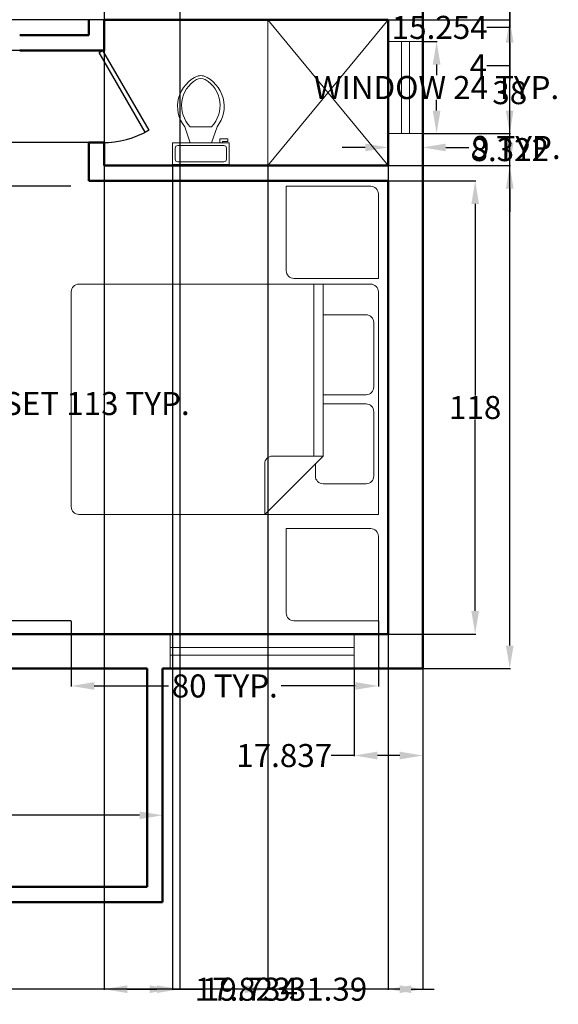
# Model space of a CAD drawing. Units: inches. Extents: x -8 to 300, y -428 to 46.
# Tile 2 of 4: x 160 to 300, y -428 to -172. Entities that reach past the tile are written whole.
import ezdxf

# ---------------------------------------------------------------- set-up
doc = ezdxf.new("R2010")
doc.units = ezdxf.units.IN
doc.header["$MEASUREMENT"] = 0
for name, color, linetype, lineweight in [('A-ANNO-DIMS', 2, 'Continuous', 18), ('A-DOOR', 3, 'Continuous', 25), ('A-FLOR-FIXT', 9, 'Continuous', 18), ('A-FURN', 8, 'Continuous', 18), ('A-GLAZ', 4, 'Continuous', 18), ('A-WALL', 7, 'Continuous', 50)]:
    doc.layers.add(name, color=color, linetype=linetype, lineweight=lineweight)
doc.styles.get("Standard").update_dxf_attribs({"font": 'arial.ttf'})
doc.dimstyles.get("Standard").update_dxf_attribs({"dimtxt": 6, "dimasz": 6, "dimexe": 0.18, "dimexo": 0.0625, "dimgap": 0.09, "dimtad": 0, "dimtih": 1, "dimtoh": 1, "dimdec": 0, "dimzin": 0, "dimdsep": 46, "dimlunit": 4, "dimtxsty": 'Standard', "dimcen": 0.09, "dimadec": 0, "dimazin": 0, "dimtfac": 1, "dimtdec": 0, "dimtofl": 0, "dimtmove": 0, "dimatfit": 3, "dimfxl": 1, "dimtolj": 1, "dimtzin": 0, "dimarcsym": 0})

# ---------------------------------------------------------------- blocks, each defined once
blk = doc.blocks.new('*U11')
for p, q in [((0, 0), (0, -6)), ((40, 0), (40, -6))]:
    blk.add_line(p, q)
blk.add_lwpolyline([(0, 0), (34.64, 20), (35.52, 18.48), (0.87, -1.52)], close=True)
blk.add_arc((0, 0), 40, 0, 30)
blk = doc.blocks.new('Toilet - top')
for p, q in [((9.5, -6), (9.5, -2)), ((-10, -8.5), (-8, -8.5)), ((-10, -9.5), (-10, -8.5)), ((-7, -9.5), (-10, -9.5)), ((-8, -8.5), (-8, -8)), ((-7, -8), (-7, -9.5)), ((-4, -8), (-6, -14)), ((4, -8), (6, -14)), ((4, -14), (-4, -14))]:
    blk.add_line(p, q)
blk.add_lwpolyline([(10.5, -8), (10.5, 0), (-10.5, 0), (-10.5, -8)], close=True)
for points in [[(-9.5, -2), (-9.5, -6)], [(8.5, -1), (-8.5, -1)], [(-8.5, -7), (8.5, -7)]]:
    blk.add_lwpolyline(points)
for centre, radius, start, end in [((-8.62, -1.88), 0.884, 81.8699, 188.1301), ((8.62, -1.88), 0.884, 351.8699, 98.1301), ((-8.62, -6.12), 0.884, 171.8699, 278.1301), ((8.62, -6.12), 0.884, 261.8699, 8.1301), ((3.52, -21.58), 12.17, 141.4691, 247.9714), ((4.2, -21.82), 11.33, 136.3677, 238.9468), ((-3.52, -21.58), 12.17, 292.0284, 38.5307), ((-4.2, -21.82), 11.33, 301.053, 43.6321), ((0, -27.88), 4, 245.7318, 294.2682), ((0, -29), 4, 254.8605, 285.1395)]:
    blk.add_arc(centre, radius, start, end)
blk = doc.blocks.new('Bed - Queen')
for p, q in [((2, 0), (60, 0)), ((60, 0), (60, -78)), ((0, -78), (0, -2)), ((10, -1.2), (26.8, -1.2)), ((33.2, -1.2), (50, -1.2)), ((8, -14.4), (8, -3.2)), ((28.8, -3.2), (28.8, -14.4)), ((31.2, -14.4), (31.2, -3.2)), ((52, -3.2), (52, -14.4)), ((0, -14.4), (44.8, -14.4)), ((60, -29.6), (44.8, -14.4)), ((44.8, -14.4), (44.8, -27.6)), ((44.8, -16.8), (0, -16.8)), ((50, -16.4), (46.8, -16.4)), ((46.8, -29.6), (60, -29.6)), ((58, -80), (2, -80))]:
    blk.add_line(p, q)
for points in [[(-1.48, 0), (-23.48, 0, 0.414214), (-25.48, -2), (-25.48, -24), (-3.48, -24, 0.414214), (-1.48, -22)], [(65.69, 0), (87.69, 0), (87.69, -22, -0.414214), (85.69, -24), (63.69, -24), (63.69, -2, -0.414214)]]:
    blk.add_lwpolyline(points, format="xyb", close=True)
for centre, start, end in [((2, -2), 90, 180), ((10, -3.2), 90, 180), ((26.8, -3.2), 0, 90), ((33.2, -3.2), 90, 180), ((50, -3.2), 0, 90), ((50, -14.4), 270, 0), ((46.8, -27.6), 180, 270), ((2, -78), 180, 270), ((58, -78), 270, 0)]:
    blk.add_arc(centre, 2, start, end)
blk = doc.blocks.new('WIN-48IN')
for p, q in [((0, 0), (0, 9)), ((48, 9), (48, 0)), ((0, 5.5), (48, 5.5)), ((0, 3.5), (48, 3.5))]:
    blk.add_line(p, q)
blk = doc.blocks.new('WIN-24IN')
for p, q in [((0, 24), (9, 24)), ((3.5, 24), (3.5, 0)), ((5.5, 24), (5.5, 0)), ((9, 0), (0, 0))]:
    blk.add_line(p, q)
blk = doc.blocks.new('*D17')
at = {"layer": 'A-ANNO-DIMS', "color": 0, "lineweight": -2, "transparency": 16777216}
for p, q in [((173.24, -215.1), (156.15, -215.1)), ((156.33, -221.1), (156.33, -268.3)), ((156.33, -322.26), (156.33, -275.06)), ((173.24, -328.26), (156.15, -328.26))]:
    blk.add_line(p, q, dxfattribs=at)
at = {"layer": 'A-ANNO-DIMS', "color": 0, "transparency": 16777216}
for points in [[(155.33, -221.1), (157.33, -221.1), (156.33, -215.1)], [(155.33, -322.26), (157.33, -322.26), (156.33, -328.26)]]:
    blk.add_solid(points, dxfattribs=at)
at = {"layer": 'Defpoints', "color": 0, "transparency": 16777216}
for p in [(173.3, -215.1), (156.33, -328.26), (173.3, -328.26)]:
    blk.add_point(p, dxfattribs=at)
at = {"layer": 'A-ANNO-DIMS', "color": 0, "transparency": 16777216, "insert": (156.33, -271.68), "char_height": 6, "attachment_point": 5}
blk.add_mtext('\\A1;QUEEN BED SET 113 TYP.', dxfattribs=at)
blk = doc.blocks.new('*D18')
at = {"layer": 'A-ANNO-DIMS', "color": 0, "lineweight": -2, "transparency": 16777216}
for p, q in [((173.3, -328.32), (173.3, -345.42)), ((253.3, -328.32), (253.3, -345.42)), ((179.3, -345.24), (198.61, -345.24)), ((247.3, -345.24), (228, -345.24))]:
    blk.add_line(p, q, dxfattribs=at)
at = {"layer": 'A-ANNO-DIMS', "color": 0, "transparency": 16777216}
for points in [[(179.3, -344.24), (179.3, -346.24), (173.3, -345.24)], [(247.3, -344.24), (247.3, -346.24), (253.3, -345.24)]]:
    blk.add_solid(points, dxfattribs=at)
at = {"layer": 'Defpoints', "color": 0, "transparency": 16777216}
for p in [(173.3, -328.26), (253.3, -328.26), (253.3, -345.24)]:
    blk.add_point(p, dxfattribs=at)
at = {"layer": 'A-ANNO-DIMS', "color": 0, "transparency": 16777216, "insert": (213.3, -345.24), "char_height": 6, "attachment_point": 5}
blk.add_mtext('\\A1;80 TYP.', dxfattribs=at)
blk = doc.blocks.new('*D21')
at = {"layer": 'A-ANNO-DIMS', "color": 0, "lineweight": -2, "transparency": 16777216}
for p, q in [((264.94, -177.38), (268.66, -177.38)), ((268.48, -183.38), (268.48, -186.19)), ((268.48, -195.38), (268.48, -192.58)), ((264.94, -201.38), (268.66, -201.38))]:
    blk.add_line(p, q, dxfattribs=at)
at = {"layer": 'A-ANNO-DIMS', "color": 0, "transparency": 16777216}
for points in [[(267.48, -183.38), (269.48, -183.38), (268.48, -177.38)], [(267.48, -195.38), (269.48, -195.38), (268.48, -201.38)]]:
    blk.add_solid(points, dxfattribs=at)
at = {"layer": 'Defpoints', "color": 0, "transparency": 16777216}
for p in [(264.88, -177.38), (268.48, -177.38), (264.88, -201.38)]:
    blk.add_point(p, dxfattribs=at)
at = {"layer": 'A-ANNO-DIMS', "color": 0, "transparency": 16777216, "insert": (268.48, -189.38), "char_height": 6, "attachment_point": 5}
blk.add_mtext('\\A1;WINDOW 24 TYP.', dxfattribs=at)
blk = doc.blocks.new('*D22')
at = {"layer": 'A-ANNO-DIMS', "color": 0, "lineweight": -2, "transparency": 16777216}
for p, q in [((255.88, -201.45), (255.88, -205.16)), ((264.88, -201.45), (264.88, -205.16)), ((249.88, -204.98), (243.88, -204.98)), ((270.88, -204.98), (276.88, -204.98))]:
    blk.add_line(p, q, dxfattribs=at)
at = {"layer": 'A-ANNO-DIMS', "color": 0, "transparency": 16777216}
for points in [[(249.88, -203.98), (249.88, -205.98), (255.88, -204.98)], [(270.88, -203.98), (270.88, -205.98), (264.88, -204.98)]]:
    blk.add_solid(points, dxfattribs=at)
at = {"layer": 'Defpoints', "color": 0, "transparency": 16777216}
for p in [(255.88, -201.38), (264.88, -201.38), (264.88, -204.98)]:
    blk.add_point(p, dxfattribs=at)
at = {"layer": 'A-ANNO-DIMS', "color": 0, "transparency": 16777216, "insert": (289.24, -204.98), "char_height": 6, "attachment_point": 5}
blk.add_mtext('\\A1;9 TYP.', dxfattribs=at)
blk = doc.blocks.new('*D31')
at = {"layer": 'A-ANNO-DIMS', "color": 0, "lineweight": -2, "transparency": 16777216}
for p, q in [((24.88, -340.77), (24.88, -424.4)), ((264.88, -340.77), (264.88, -424.4)), ((30.88, -424.22), (138.12, -424.22)), ((258.88, -424.22), (151.64, -424.22))]:
    blk.add_line(p, q, dxfattribs=at)
at = {"layer": 'A-ANNO-DIMS', "color": 0, "transparency": 16777216}
for points in [[(30.88, -423.22), (30.88, -425.22), (24.88, -424.22)], [(258.88, -423.22), (258.88, -425.22), (264.88, -424.22)]]:
    blk.add_solid(points, dxfattribs=at)
at = {"layer": 'Defpoints', "color": 0, "transparency": 16777216}
for p in [(24.88, -340.71), (264.88, -340.71), (264.88, -424.22)]:
    blk.add_point(p, dxfattribs=at)
at = {"layer": 'A-ANNO-DIMS', "color": 0, "transparency": 16777216, "insert": (144.88, -424.22), "char_height": 6, "attachment_point": 5}
blk.add_mtext('\\A1;240', dxfattribs=at)
blk = doc.blocks.new('*D33')
at = {"layer": 'A-ANNO-DIMS', "color": 0, "lineweight": -2, "transparency": 16777216}
for p, q in [((264.94, 19.29), (287.71, 19.29)), ((287.53, 13.29), (287.53, -157.55)), ((287.53, -334.71), (287.53, -163.86)), ((264.94, -340.71), (287.71, -340.71))]:
    blk.add_line(p, q, dxfattribs=at)
at = {"layer": 'A-ANNO-DIMS', "color": 0, "transparency": 16777216}
for points in [[(286.53, 13.29), (288.53, 13.29), (287.53, 19.29)], [(286.53, -334.71), (288.53, -334.71), (287.53, -340.71)]]:
    blk.add_solid(points, dxfattribs=at)
at = {"layer": 'Defpoints', "color": 0, "transparency": 16777216}
for p in [(264.88, 19.29), (264.88, -340.71), (287.53, -340.71)]:
    blk.add_point(p, dxfattribs=at)
at = {"layer": 'A-ANNO-DIMS', "color": 0, "transparency": 16777216, "insert": (287.53, -160.71), "char_height": 6, "attachment_point": 5}
blk.add_mtext('\\A1;360', dxfattribs=at)
blk = doc.blocks.new('*D34')
at = {"layer": 'A-ANNO-DIMS', "color": 0, "lineweight": -2, "transparency": 16777216}
for p, q in [((81.19, -401.51), (81.19, -378.74)), ((87.19, -378.92), (129.21, -378.92)), ((191.09, -378.92), (149.08, -378.92)), ((197.09, -401.51), (197.09, -378.74))]:
    blk.add_line(p, q, dxfattribs=at)
at = {"layer": 'A-ANNO-DIMS', "color": 0, "transparency": 16777216}
for points in [[(87.19, -377.92), (87.19, -379.92), (81.19, -378.92)], [(191.09, -377.92), (191.09, -379.92), (197.09, -378.92)]]:
    blk.add_solid(points, dxfattribs=at)
at = {"layer": 'Defpoints', "color": 0, "transparency": 16777216}
for p in [(197.09, -378.92), (81.19, -401.57), (197.09, -401.57)]:
    blk.add_point(p, dxfattribs=at)
at = {"layer": 'A-ANNO-DIMS', "color": 0, "transparency": 16777216, "insert": (139.14, -378.92), "char_height": 6, "attachment_point": 5}
blk.add_mtext('\\A1;115.9', dxfattribs=at)
blk = doc.blocks.new('*D40')
at = {"layer": 'A-ANNO-DIMS', "color": 0, "lineweight": -2, "transparency": 16777216}
for p, q in [((255.94, -213.71), (278.71, -213.71)), ((278.53, -219.71), (278.53, -269.55)), ((278.53, -325.71), (278.53, -275.86)), ((255.94, -331.71), (278.71, -331.71))]:
    blk.add_line(p, q, dxfattribs=at)
at = {"layer": 'A-ANNO-DIMS', "color": 0, "transparency": 16777216}
for points in [[(277.53, -219.71), (279.53, -219.71), (278.53, -213.71)], [(277.53, -325.71), (279.53, -325.71), (278.53, -331.71)]]:
    blk.add_solid(points, dxfattribs=at)
at = {"layer": 'Defpoints', "color": 0, "transparency": 16777216}
for p in [(255.88, -213.71), (255.88, -331.71), (278.53, -331.71)]:
    blk.add_point(p, dxfattribs=at)
at = {"layer": 'A-ANNO-DIMS', "color": 0, "transparency": 16777216, "insert": (278.53, -272.71), "char_height": 6, "attachment_point": 5}
blk.add_mtext('\\A1;118', dxfattribs=at)
blk = doc.blocks.new('*D50')
at = {"layer": 'A-ANNO-DIMS', "color": 0, "lineweight": -2, "transparency": 16777216}
for p, q in [((247.04, -340.77), (247.04, -363.54)), ((264.88, -340.77), (264.88, -363.54)), ((247.04, -363.36), (241.04, -363.36)), ((258.88, -363.36), (253.04, -363.36))]:
    blk.add_line(p, q, dxfattribs=at)
at = {"layer": 'A-ANNO-DIMS', "color": 0, "transparency": 16777216}
for points in [[(253.04, -362.36), (253.04, -364.36), (247.04, -363.36)], [(258.88, -362.36), (258.88, -364.36), (264.88, -363.36)]]:
    blk.add_solid(points, dxfattribs=at)
at = {"layer": 'Defpoints', "color": 0, "transparency": 16777216}
for p in [(247.04, -340.71), (264.88, -340.71), (247.04, -363.36)]:
    blk.add_point(p, dxfattribs=at)
at = {"layer": 'A-ANNO-DIMS', "color": 0, "transparency": 16777216, "insert": (228.78, -363.36), "char_height": 6, "attachment_point": 5}
blk.add_mtext('\\A1;17.837', dxfattribs=at)
blk = doc.blocks.new('*D54')
at = {"layer": 'A-ANNO-DIMS', "color": 0, "lineweight": -2, "transparency": 16777216}
for p, q in [((255.94, -171.71), (287.71, -171.71)), ((287.53, -177.71), (287.53, -187.55)), ((287.53, -203.71), (287.53, -193.86)), ((255.94, -209.71), (287.71, -209.71))]:
    blk.add_line(p, q, dxfattribs=at)
at = {"layer": 'A-ANNO-DIMS', "color": 0, "transparency": 16777216}
for points in [[(286.53, -177.71), (288.53, -177.71), (287.53, -171.71)], [(286.53, -203.71), (288.53, -203.71), (287.53, -209.71)]]:
    blk.add_solid(points, dxfattribs=at)
at = {"layer": 'Defpoints', "color": 0, "transparency": 16777216}
for p in [(255.88, -171.71), (255.88, -209.71), (287.53, -209.71)]:
    blk.add_point(p, dxfattribs=at)
at = {"layer": 'A-ANNO-DIMS', "color": 0, "transparency": 16777216, "insert": (287.53, -190.71), "char_height": 6, "attachment_point": 5}
blk.add_mtext('\\A1;38', dxfattribs=at)
blk = doc.blocks.new('*D55')
at = {"layer": 'A-ANNO-DIMS', "color": 0, "lineweight": -2, "transparency": 16777216}
for p, q in [((287.53, -161.71), (287.53, -155.71)), ((255.94, -167.71), (287.71, -167.71)), ((255.94, -171.71), (287.71, -171.71)), ((287.53, -177.71), (287.53, -183.71)), ((287.53, -183.71), (281.53, -183.71))]:
    blk.add_line(p, q, dxfattribs=at)
at = {"layer": 'A-ANNO-DIMS', "color": 0, "transparency": 16777216}
for points in [[(286.53, -161.71), (288.53, -161.71), (287.53, -167.71)], [(286.53, -177.71), (288.53, -177.71), (287.53, -171.71)]]:
    blk.add_solid(points, dxfattribs=at)
at = {"layer": 'Defpoints', "color": 0, "transparency": 16777216}
for p in [(255.88, -167.71), (255.88, -171.71), (287.53, -171.71)]:
    blk.add_point(p, dxfattribs=at)
at = {"layer": 'A-ANNO-DIMS', "color": 0, "transparency": 16777216, "insert": (279.36, -183.71), "char_height": 6, "attachment_point": 5}
blk.add_mtext('\\A1;4', dxfattribs=at)
blk = doc.blocks.new('*D58')
at = {"layer": 'A-ANNO-DIMS', "color": 0, "lineweight": -2, "transparency": 16777216}
for p, q in [((2.225934, -165.706734), (2.225934, -159.706734)), ((181.813434, -171.706734), (2.045934, -171.706734)), ((177.813434, -179.706734), (2.045934, -179.706734)), ((2.225934, -185.706734), (2.225934, -191.706734))]:
    blk.add_line(p, q, dxfattribs=at)
at = {"layer": 'A-ANNO-DIMS', "color": 0, "transparency": 16777216}
for points in [[(1.225934, -165.706734), (3.225934, -165.706734), (2.225934, -171.706734)], [(1.225934, -185.706734), (3.225934, -185.706734), (2.225934, -179.706734)]]:
    blk.add_solid(points, dxfattribs=at)
at = {"layer": 'Defpoints', "color": 0, "transparency": 16777216}
for p in [(2.225934, -171.706734), (181.875934, -171.706734), (177.875934, -179.706734)]:
    blk.add_point(p, dxfattribs=at)
at = {"layer": 'A-ANNO-DIMS', "color": 0, "transparency": 16777216, "insert": (2.225934, -175.706734), "char_height": 6, "attachment_point": 5}
blk.add_mtext('\\A1;8', dxfattribs=at)
blk = doc.blocks.new('*D59')
at = {"layer": 'A-ANNO-DIMS', "color": 0, "lineweight": -2, "transparency": 16777216}
for p, q in [((177.81, -179.71), (2.05, -179.71)), ((2.23, -185.71), (2.23, -188.6)), ((2.23, -197.71), (2.23, -194.81)), ((177.81, -203.71), (2.05, -203.71))]:
    blk.add_line(p, q, dxfattribs=at)
at = {"layer": 'A-ANNO-DIMS', "color": 0, "transparency": 16777216}
for points in [[(1.23, -185.71), (3.23, -185.71), (2.23, -179.71)], [(1.23, -197.71), (3.23, -197.71), (2.23, -203.71)]]:
    blk.add_solid(points, dxfattribs=at)
at = {"layer": 'Defpoints', "color": 0, "transparency": 16777216}
for p in [(2.23, -179.71), (177.88, -179.71), (177.88, -203.71)]:
    blk.add_point(p, dxfattribs=at)
at = {"layer": 'A-ANNO-DIMS', "color": 0, "transparency": 16777216, "insert": (2.23, -191.71), "char_height": 6, "attachment_point": 5}
blk.add_mtext('\\A1;24', dxfattribs=at)
blk = doc.blocks.new('*D60')
at = {"layer": 'A-ANNO-DIMS', "color": 0, "lineweight": -2, "transparency": 16777216}
for p, q in [((224.485356, -209.769234), (224.485356, -424.397677)), ((255.875934, -209.769234), (255.875934, -424.397677)), ((218.485356, -424.217677), (212.485356, -424.217677)), ((261.875934, -424.217677), (267.875934, -424.217677))]:
    blk.add_line(p, q, dxfattribs=at)
at = {"layer": 'A-ANNO-DIMS', "color": 0, "transparency": 16777216}
for points in [[(218.485356, -423.217677), (218.485356, -425.217677), (224.485356, -424.217677)], [(261.875934, -423.217677), (261.875934, -425.217677), (255.875934, -424.217677)]]:
    blk.add_solid(points, dxfattribs=at)
at = {"layer": 'Defpoints', "color": 0, "transparency": 16777216}
for p in [(224.485356, -209.706734), (255.875934, -209.706734), (224.485356, -424.217677)]:
    blk.add_point(p, dxfattribs=at)
at = {"layer": 'A-ANNO-DIMS', "color": 0, "transparency": 16777216, "insert": (240.180645, -424.217677), "char_height": 6, "attachment_point": 5}
blk.add_mtext('\\A1;31.39', dxfattribs=at)
blk = doc.blocks.new('*D61')
at = {"layer": 'A-ANNO-DIMS', "color": 0, "lineweight": -2, "transparency": 16777216}
for p, q in [((264.94, -152.45), (287.71, -152.45)), ((287.53, -158.45), (287.53, -161.71)), ((255.94, -167.71), (287.71, -167.71)), ((287.53, -167.71), (287.53, -173.71)), ((287.53, -173.71), (281.53, -173.71))]:
    blk.add_line(p, q, dxfattribs=at)
at = {"layer": 'A-ANNO-DIMS', "color": 0, "transparency": 16777216}
for points in [[(286.53, -158.45), (288.53, -158.45), (287.53, -152.45)], [(286.53, -161.71), (288.53, -161.71), (287.53, -167.71)]]:
    blk.add_solid(points, dxfattribs=at)
at = {"layer": 'Defpoints', "color": 0, "transparency": 16777216}
for p in [(264.88, -152.45), (255.88, -167.71), (287.53, -167.71)]:
    blk.add_point(p, dxfattribs=at)
at = {"layer": 'A-ANNO-DIMS', "color": 0, "transparency": 16777216, "insert": (269.28, -173.71), "char_height": 6, "attachment_point": 5}
blk.add_mtext('\\A1;15.254', dxfattribs=at)
blk = doc.blocks.new('*D62')
at = {"layer": 'A-ANNO-DIMS', "color": 0, "lineweight": -2, "transparency": 16777216}
for p, q in [((287.53, -195.38), (287.53, -189.38)), ((264.94, -201.38), (287.71, -201.38)), ((255.94, -209.71), (287.71, -209.71)), ((287.53, -215.71), (287.53, -221.71))]:
    blk.add_line(p, q, dxfattribs=at)
at = {"layer": 'A-ANNO-DIMS', "color": 0, "transparency": 16777216}
for points in [[(286.53, -195.38), (288.53, -195.38), (287.53, -201.38)], [(286.53, -215.71), (288.53, -215.71), (287.53, -209.71)]]:
    blk.add_solid(points, dxfattribs=at)
at = {"layer": 'Defpoints', "color": 0, "transparency": 16777216}
for p in [(264.88, -201.38), (255.88, -209.71), (287.53, -209.71)]:
    blk.add_point(p, dxfattribs=at)
at = {"layer": 'A-ANNO-DIMS', "color": 0, "transparency": 16777216, "insert": (287.53, -205.55), "char_height": 6, "attachment_point": 5}
blk.add_mtext('\\A1;8.322', dxfattribs=at)
blk = doc.blocks.new('*D63')
at = {"layer": 'A-ANNO-DIMS', "color": 0, "lineweight": -2, "transparency": 16777216}
for p, q in [((181.88, -111.77), (181.88, -424.4)), ((201.61, -113.22), (201.61, -424.4)), ((187.88, -424.22), (195.61, -424.22)), ((201.61, -424.22), (207.61, -424.22))]:
    blk.add_line(p, q, dxfattribs=at)
at = {"layer": 'A-ANNO-DIMS', "color": 0, "transparency": 16777216}
for points in [[(187.88, -423.22), (187.88, -425.22), (181.88, -424.22)], [(195.61, -423.22), (195.61, -425.22), (201.61, -424.22)]]:
    blk.add_solid(points, dxfattribs=at)
at = {"layer": 'Defpoints', "color": 0, "transparency": 16777216}
for p in [(181.88, -111.71), (201.61, -113.16), (201.61, -424.22)]:
    blk.add_point(p, dxfattribs=at)
at = {"layer": 'A-ANNO-DIMS', "color": 0, "transparency": 16777216, "insert": (219.86, -424.22), "char_height": 6, "attachment_point": 5}
blk.add_mtext('\\A1;19.734', dxfattribs=at)
blk = doc.blocks.new('*D64')
at = {"layer": 'A-ANNO-DIMS', "color": 0, "lineweight": -2, "transparency": 16777216}
for p, q in [((181.88, -209.77), (181.88, -424.4)), ((199.7, -209.48), (199.7, -424.4)), ((187.88, -424.22), (193.7, -424.22)), ((199.7, -424.22), (205.7, -424.22))]:
    blk.add_line(p, q, dxfattribs=at)
at = {"layer": 'A-ANNO-DIMS', "color": 0, "transparency": 16777216}
for points in [[(187.88, -423.22), (187.88, -425.22), (181.88, -424.22)], [(193.7, -423.22), (193.7, -425.22), (199.7, -424.22)]]:
    blk.add_solid(points, dxfattribs=at)
at = {"layer": 'Defpoints', "color": 0, "transparency": 16777216}
for p in [(181.88, -209.71), (199.7, -209.41), (199.7, -424.22)]:
    blk.add_point(p, dxfattribs=at)
at = {"layer": 'A-ANNO-DIMS', "color": 0, "transparency": 16777216, "insert": (217.96, -424.22), "char_height": 6, "attachment_point": 5}
blk.add_mtext('\\A1;17.823', dxfattribs=at)

msp = doc.modelspace()

# ---------------------------------------------------------------- linework, layer by layer
at = {"layer": 'A-FLOR-FIXT'}
for p, q in [((224.4854, -171.7067), (255.8759, -209.7067)), ((255.8759, -171.7067), (224.4854, -209.7067))]:
    msp.add_line(p, q, dxfattribs=at)
msp.add_lwpolyline([(224.4854, -171.7067), (224.4854, -209.7067), (255.8759, -209.7067), (255.8759, -171.7067)], dxfattribs=at)
at = {"layer": 'A-WALL'}
for p, q in [((177.8759, -171.7067), (177.8759, -175.7067)), ((181.8759, -171.7067), (255.8759, -171.7067)), ((181.8759, -171.7067), (181.8759, -179.7067)), ((255.8759, -171.7067), (255.8759, -209.7067)), ((159.8759, -175.7067), (177.8759, -175.7067)), ((177.8759, -179.7067), (159.8759, -179.7067)), ((177.8759, -179.7067), (181.8759, -179.7067)), ((177.8759, -203.7067), (181.8759, -203.7067)), ((177.8759, -203.7067), (177.8759, -209.7067)), ((181.8759, -203.7067), (181.8759, -209.7067)), ((177.8759, -209.7067), (177.8759, -213.7067)), ((255.8759, -209.7067), (181.8759, -209.7067)), ((255.8759, -213.7067), (177.8759, -213.7067)), ((255.8759, -213.7067), (255.8759, -331.7067)), ((255.8759, -331.7067), (123.8759, -331.7067)), ((85.1915, -340.7067), (193.0947, -340.7067)), ((193.0947, -340.7067), (193.0947, -397.5677)), ((197.0947, -340.7067), (197.0947, -401.5677)), ((193.0947, -397.5677), (85.1915, -397.5677)), ((197.0947, -401.5677), (81.1915, -401.5677))]:
    msp.add_line(p, q, dxfattribs=at)
msp.add_lwpolyline([(39.8759, -340.7067), (24.8759, -340.7067), (24.8759, 19.2933), (264.8759, 19.2933), (264.8759, -340.7067), (197.0947, -340.7067)], dxfattribs=at)

# ---------------------------------------------------------------- block references
at = {"layer": 'A-DOOR', "xscale": 0.6, "yscale": 0.6, "zscale": 0.6, "rotation": 270}
msp.add_blockref('*U11', (181.4759, -179.7067), dxfattribs=at)
at = {"layer": 'A-FLOR-FIXT', "xscale": 0.7015592468028999, "yscale": 0.7015592468028999, "zscale": 0.7015592468028999, "rotation": 180.0000000000001}
msp.add_blockref('Toilet - top', (207.0654, -209.413), dxfattribs=at)
at = {"layer": 'A-FURN', "rotation": 270}
msp.add_blockref('Bed - Queen', (253.3035, -240.5723), dxfattribs=at)
at = {"layer": 'A-GLAZ'}
for name, p in [('WIN-24IN', (255.876, -201.3847)), ('WIN-48IN', (199.0391, -340.7069))]:
    msp.add_blockref(name, p, dxfattribs=at)

# ---------------------------------------------------------------- dimensions: what is measured, and where the dimension line sits
at = {"layer": 'A-ANNO-DIMS'}
for base, p1, p2, angle, override, picture, middle in [((287.5259, -340.7067), (264.8759, 19.2933), (264.8759, -340.7067), 90, {"dimdec": 0, "dimlfac": 1, "dimrnd": 0, "dimzin": 0, "dimdsep": 46, "dimlunit": 2}, '*D33', (287.5259, -160.7067)), ((287.5259, -167.7067), (264.8759, -152.453), (255.8759, -167.7067), 90, {"dimdec": 3, "dimlfac": 1, "dimrnd": 0, "dimzin": 0, "dimdsep": 46, "dimlunit": 2}, '*D61', (269.2763, -173.7067)), ((287.5259, -171.7067), (255.8759, -167.7067), (255.8759, -171.7067), 90, {"dimdec": 0, "dimlfac": 1, "dimrnd": 0, "dimzin": 0, "dimdsep": 46, "dimlunit": 2}, '*D55', (279.3609, -183.7067)), ((2.2259, -171.7067), (177.8759, -179.7067), (181.8759, -171.7067), 90, {"dimdec": 0, "dimlfac": 1, "dimrnd": 0, "dimzin": 0, "dimdsep": 46, "dimlunit": 2}, '*D58', (2.2259, -175.7067)), ((287.5259, -209.7067), (255.8759, -171.7067), (255.8759, -209.7067), 90, {"dimdec": 0, "dimlfac": 1, "dimrnd": 0, "dimzin": 0, "dimdsep": 46, "dimlunit": 2}, '*D54', (287.5259, -190.7067)), ((2.2259, -179.7067), (177.8759, -203.7067), (177.8759, -179.7067), 90, {"dimdec": 0, "dimlfac": 1, "dimrnd": 0, "dimzin": 0, "dimdsep": 46, "dimlunit": 2}, '*D59', (2.2259, -191.7067)), ((287.5259, -209.7067), (264.8759, -201.3847), (255.8759, -209.7067), 90, {"dimdec": 3, "dimlfac": 1, "dimrnd": 0, "dimzin": 0, "dimdsep": 46, "dimlunit": 2}, '*D62', (287.5259, -205.5457)), ((278.5259, -331.7067), (255.8759, -213.7067), (255.8759, -331.7067), 270, {"dimdec": 0, "dimlfac": 1, "dimrnd": 0, "dimzin": 0, "dimdsep": 46, "dimlunit": 2}, '*D40', (278.5259, -272.7067)), ((247.0393, -363.3567), (264.8759, -340.7067), (247.0393, -340.7067), 180, {"dimdec": 3, "dimlfac": 1, "dimrnd": 0, "dimzin": 0, "dimdsep": 46, "dimlunit": 2}, '*D50', (228.7774, -363.3567))]:
    dim = msp.add_linear_dim(base=base, p1=p1, p2=p2, angle=angle, dimstyle='Standard', override=override, dxfattribs=at)
    dim.commit()
    dim.dimension.update_dxf_attribs({"geometry": picture, "text_midpoint": middle})
for base, p1, p2, override, picture, middle in [((201.6099, -424.2177), (181.8759, -111.7067), (201.6099, -113.157), {"dimdec": 3, "dimlfac": 1, "dimrnd": 0, "dimzin": 0, "dimdsep": 46, "dimlunit": 2}, '*D63', (219.8595, -424.2177)), ((199.6991, -424.2177), (181.8759, -209.7067), (199.6991, -209.413), {"dimdec": 3, "dimlfac": 1, "dimrnd": 0, "dimzin": 0, "dimdsep": 46, "dimlunit": 2}, '*D64', (217.961, -424.2177)), ((224.4854, -424.2177), (255.8759, -209.7067), (224.4854, -209.7067), {"dimdec": 2, "dimlfac": 1, "dimrnd": 0, "dimzin": 0, "dimdsep": 46, "dimlunit": 2}, '*D60', (240.1806, -424.2177)), ((264.8759, -424.2177), (24.8759, -340.7067), (264.8759, -340.7067), {"dimdec": 0, "dimlfac": 1, "dimrnd": 0, "dimzin": 0, "dimdsep": 46, "dimlunit": 2}, '*D31', (144.8759, -424.2177)), ((197.0947, -378.9177), (81.1915, -401.5677), (197.0947, -401.5677), {"dimdec": 1, "dimlfac": 1, "dimrnd": 0, "dimzin": 0, "dimdsep": 46, "dimlunit": 2}, '*D34', (139.1431, -378.9177))]:
    dim = msp.add_linear_dim(base=base, p1=p1, p2=p2, dimstyle='Standard', override=override, dxfattribs=at)
    dim.commit()
    dim.dimension.update_dxf_attribs({"geometry": picture, "text_midpoint": middle})
for base, p1, p2, angle, text, picture, middle in [((268.4759, -177.3847), (264.8759, -201.3847), (264.8759, -177.3847), 90, 'WINDOW <> TYP.', '*D21', (268.4759, -189.3847)), ((156.3284, -328.262), (173.3035, -215.0951), (173.3035, -328.262), 270, 'QUEEN BED SET <> TYP.', '*D17', (156.3284, -271.6785))]:
    dim = msp.add_linear_dim(base=base, p1=p1, p2=p2, angle=angle, text=text, dimstyle='Standard', override={"dimdec": 0, "dimlfac": 1, "dimrnd": 0, "dimzin": 0, "dimdsep": 46, "dimlunit": 2}, dxfattribs=at)
    dim.commit()
    dim.dimension.update_dxf_attribs({"geometry": picture, "text_midpoint": middle})
for base, p1, p2, picture, middle in [((264.8759, -204.9847), (255.8759, -201.3847), (264.8759, -201.3847), '*D22', (289.2381, -204.9847)), ((253.3035, -345.237), (173.3035, -328.262), (253.3035, -328.262), '*D18', (213.3035, -345.237))]:
    dim = msp.add_linear_dim(base=base, p1=p1, p2=p2, text='<> TYP.', dimstyle='Standard', override={"dimdec": 0, "dimlfac": 1, "dimrnd": 0, "dimzin": 0, "dimdsep": 46, "dimlunit": 2}, dxfattribs=at)
    dim.commit()
    dim.dimension.update_dxf_attribs({"geometry": picture, "text_midpoint": middle})

doc.saveas('drawing.dxf')
